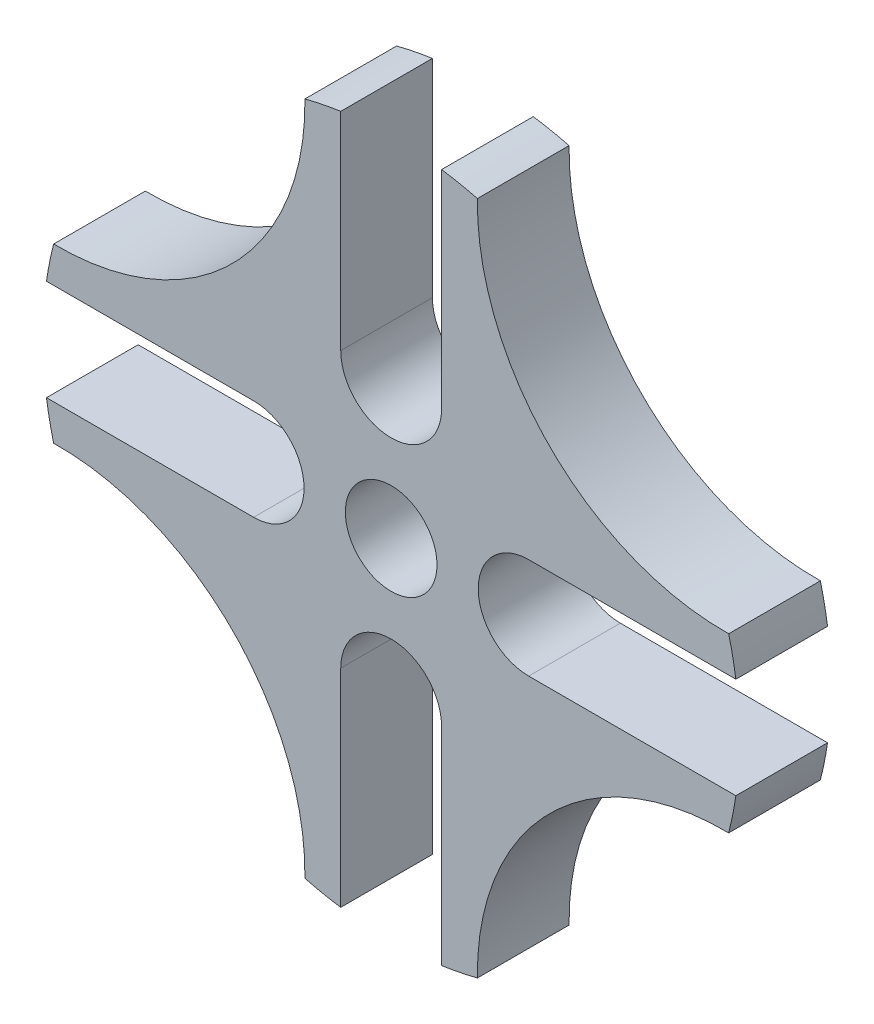
ISO-10303-21;
HEADER;
FILE_DESCRIPTION(('STEP AP214'),'2;1');
FILE_NAME('part.step','',(''),(''),'','','');
FILE_SCHEMA(('AUTOMOTIVE_DESIGN { 1 0 10303 214 1 1 1 1 }'));
ENDSEC;
DATA;
#1=APPLICATION_CONTEXT('core data for automotive mechanical design processes');
#2=APPLICATION_PROTOCOL_DEFINITION('international standard','automotive_design',2000,#1);
#3=PRODUCT_CONTEXT('',#1,'mechanical');
#4=PRODUCT('Part','Part','',(#3));
#5=PRODUCT_RELATED_PRODUCT_CATEGORY('part','',(#4));
#6=PRODUCT_DEFINITION_FORMATION('','',#4);
#7=PRODUCT_DEFINITION_CONTEXT('part definition',#1,'design');
#8=PRODUCT_DEFINITION('design','',#6,#7);
#9=PRODUCT_DEFINITION_SHAPE('','',#8);
#10=(LENGTH_UNIT() NAMED_UNIT(*) SI_UNIT(.MILLI.,.METRE.));
#11=(NAMED_UNIT(*) PLANE_ANGLE_UNIT() SI_UNIT($,.RADIAN.));
#12=(NAMED_UNIT(*) SI_UNIT($,.STERADIAN.) SOLID_ANGLE_UNIT());
#13=UNCERTAINTY_MEASURE_WITH_UNIT(LENGTH_MEASURE(1.E-05),#10,'distance_accuracy_value','');
#14=(GEOMETRIC_REPRESENTATION_CONTEXT(3) GLOBAL_UNCERTAINTY_ASSIGNED_CONTEXT((#13)) GLOBAL_UNIT_ASSIGNED_CONTEXT((#10,
#11,#12)) REPRESENTATION_CONTEXT('',''));
#15=CARTESIAN_POINT('',(0.,0.,0.));
#16=DIRECTION('',(0.,0.,1.));
#17=DIRECTION('',(1.,0.,0.));
#18=AXIS2_PLACEMENT_3D('',#15,#16,#17);
#19=CARTESIAN_POINT('',(0.,0.,10.));
#20=DIRECTION('',(0.,0.,1.));
#21=DIRECTION('',(1.,0.,0.));
#22=AXIS2_PLACEMENT_3D('',#19,#20,#21);
#23=PLANE('',#22);
#24=CARTESIAN_POINT('',(0.,0.,10.));
#25=DIRECTION('',(0.,0.,1.));
#26=DIRECTION('',(1.,0.,0.));
#27=AXIS2_PLACEMENT_3D('',#24,#25,#26);
#28=CIRCLE('',#27,38.);
#29=CARTESIAN_POINT('',(-9.40826438850213,-36.8169059155715,10.));
#30=VERTEX_POINT('',#29);
#31=CARTESIAN_POINT('',(-5.5,-37.5998670210414,10.));
#32=VERTEX_POINT('',#31);
#33=EDGE_CURVE('E276',#30,#32,#28,.T.);
#34=ORIENTED_EDGE('',*,*,#33,.T.);
#35=DIRECTION('',(0.,1.,0.));
#36=VECTOR('',#35,1.);
#37=CARTESIAN_POINT('',(-5.5,-15.,10.));
#38=LINE('',#37,#36);
#39=CARTESIAN_POINT('',(-5.5,-15.,10.));
#40=VERTEX_POINT('',#39);
#41=EDGE_CURVE('E150',#32,#40,#38,.T.);
#42=ORIENTED_EDGE('',*,*,#41,.T.);
#43=CARTESIAN_POINT('',(0.,-15.,10.));
#44=DIRECTION('',(0.,0.,-1.));
#45=DIRECTION('',(1.,0.,0.));
#46=AXIS2_PLACEMENT_3D('',#43,#44,#45);
#47=CIRCLE('',#46,5.5);
#48=CARTESIAN_POINT('',(5.5,-15.,10.));
#49=VERTEX_POINT('',#48);
#50=EDGE_CURVE('E345',#40,#49,#47,.T.);
#51=ORIENTED_EDGE('',*,*,#50,.T.);
#52=DIRECTION('',(0.,-1.,0.));
#53=VECTOR('',#52,1.);
#54=CARTESIAN_POINT('',(5.5,-15.,10.));
#55=LINE('',#54,#53);
#56=CARTESIAN_POINT('',(5.5,-37.5998670210414,10.));
#57=VERTEX_POINT('',#56);
#58=EDGE_CURVE('E363',#49,#57,#55,.T.);
#59=ORIENTED_EDGE('',*,*,#58,.T.);
#60=CARTESIAN_POINT('',(0.,0.,10.));
#61=DIRECTION('',(0.,0.,1.));
#62=DIRECTION('',(1.,0.,0.));
#63=AXIS2_PLACEMENT_3D('',#60,#61,#62);
#64=CIRCLE('',#63,38.);
#65=CARTESIAN_POINT('',(9.40826438850226,-36.8169059155714,10.));
#66=VERTEX_POINT('',#65);
#67=EDGE_CURVE('E356',#57,#66,#64,.T.);
#68=ORIENTED_EDGE('',*,*,#67,.T.);
#69=CARTESIAN_POINT('',(36.4051241273476,-36.4051241273475,10.));
#70=DIRECTION('',(0.,0.,-1.));
#71=DIRECTION('',(1.,0.,0.));
#72=AXIS2_PLACEMENT_3D('',#69,#70,#71);
#73=CIRCLE('',#72,27.);
#74=CARTESIAN_POINT('',(36.8169059155715,-9.40826438850214,10.));
#75=VERTEX_POINT('',#74);
#76=EDGE_CURVE('E357',#66,#75,#73,.T.);
#77=ORIENTED_EDGE('',*,*,#76,.T.);
#78=CARTESIAN_POINT('',(0.,0.,10.));
#79=DIRECTION('',(0.,0.,1.));
#80=DIRECTION('',(1.,0.,0.));
#81=AXIS2_PLACEMENT_3D('',#78,#79,#80);
#82=CIRCLE('',#81,38.);
#83=CARTESIAN_POINT('',(37.5998670210414,-5.5,10.));
#84=VERTEX_POINT('',#83);
#85=EDGE_CURVE('E361',#75,#84,#82,.T.);
#86=ORIENTED_EDGE('',*,*,#85,.T.);
#87=DIRECTION('',(-1.,0.,0.));
#88=VECTOR('',#87,1.);
#89=CARTESIAN_POINT('',(14.9999999999999,-5.50000000000016,10.));
#90=LINE('',#89,#88);
#91=CARTESIAN_POINT('',(14.9999999999999,-5.50000000000016,10.));
#92=VERTEX_POINT('',#91);
#93=EDGE_CURVE('E369',#84,#92,#90,.T.);
#94=ORIENTED_EDGE('',*,*,#93,.T.);
#95=CARTESIAN_POINT('',(15.,-1.57116660247941E-13,10.));
#96=DIRECTION('',(0.,0.,-1.));
#97=DIRECTION('',(1.,0.,0.));
#98=AXIS2_PLACEMENT_3D('',#95,#96,#97);
#99=CIRCLE('',#98,5.5);
#100=CARTESIAN_POINT('',(15.0000000000001,5.49999999999984,10.));
#101=VERTEX_POINT('',#100);
#102=EDGE_CURVE('E371',#92,#101,#99,.T.);
#103=ORIENTED_EDGE('',*,*,#102,.T.);
#104=DIRECTION('',(1.,0.,0.));
#105=VECTOR('',#104,1.);
#106=CARTESIAN_POINT('',(15.0000000000001,5.49999999999984,10.));
#107=LINE('',#106,#105);
#108=CARTESIAN_POINT('',(37.5998670210415,5.49999999999961,10.));
#109=VERTEX_POINT('',#108);
#110=EDGE_CURVE('E373',#101,#109,#107,.T.);
#111=ORIENTED_EDGE('',*,*,#110,.T.);
#112=CARTESIAN_POINT('',(0.,0.,10.));
#113=DIRECTION('',(0.,0.,1.));
#114=DIRECTION('',(1.,0.,0.));
#115=AXIS2_PLACEMENT_3D('',#112,#113,#114);
#116=CIRCLE('',#115,38.);
#117=CARTESIAN_POINT('',(36.8169059155714,9.40826438850227,10.));
#118=VERTEX_POINT('',#117);
#119=EDGE_CURVE('E374',#109,#118,#116,.T.);
#120=ORIENTED_EDGE('',*,*,#119,.T.);
#121=CARTESIAN_POINT('',(36.4051241273474,36.4051241273476,10.));
#122=DIRECTION('',(0.,0.,-1.));
#123=DIRECTION('',(1.,0.,0.));
#124=AXIS2_PLACEMENT_3D('',#121,#122,#123);
#125=CIRCLE('',#124,27.);
#126=CARTESIAN_POINT('',(9.40826438850214,36.8169059155715,10.));
#127=VERTEX_POINT('',#126);
#128=EDGE_CURVE('E380',#118,#127,#125,.T.);
#129=ORIENTED_EDGE('',*,*,#128,.T.);
#130=CARTESIAN_POINT('',(0.,0.,10.));
#131=DIRECTION('',(0.,0.,1.));
#132=DIRECTION('',(1.,0.,0.));
#133=AXIS2_PLACEMENT_3D('',#130,#131,#132);
#134=CIRCLE('',#133,38.);
#135=CARTESIAN_POINT('',(5.50000000000026,37.5998670210414,10.));
#136=VERTEX_POINT('',#135);
#137=EDGE_CURVE('E377',#127,#136,#134,.T.);
#138=ORIENTED_EDGE('',*,*,#137,.T.);
#139=DIRECTION('',(0.,-1.,0.));
#140=VECTOR('',#139,1.);
#141=CARTESIAN_POINT('',(5.5000000000001,15.,10.));
#142=LINE('',#141,#140);
#143=CARTESIAN_POINT('',(5.5000000000001,15.,10.));
#144=VERTEX_POINT('',#143);
#145=EDGE_CURVE('E381',#136,#144,#142,.T.);
#146=ORIENTED_EDGE('',*,*,#145,.T.);
#147=CARTESIAN_POINT('',(1.04744440165294E-13,15.,10.));
#148=DIRECTION('',(0.,0.,-1.));
#149=DIRECTION('',(1.,0.,0.));
#150=AXIS2_PLACEMENT_3D('',#147,#148,#149);
#151=CIRCLE('',#150,5.5);
#152=CARTESIAN_POINT('',(-5.49999999999989,15.,10.));
#153=VERTEX_POINT('',#152);
#154=EDGE_CURVE('E382',#144,#153,#151,.T.);
#155=ORIENTED_EDGE('',*,*,#154,.T.);
#156=DIRECTION('',(0.,1.,0.));
#157=VECTOR('',#156,1.);
#158=CARTESIAN_POINT('',(-5.49999999999989,15.,10.));
#159=LINE('',#158,#157);
#160=CARTESIAN_POINT('',(-5.49999999999974,37.5998670210415,10.));
#161=VERTEX_POINT('',#160);
#162=EDGE_CURVE('E384',#153,#161,#159,.T.);
#163=ORIENTED_EDGE('',*,*,#162,.T.);
#164=CARTESIAN_POINT('',(0.,0.,10.));
#165=DIRECTION('',(0.,0.,1.));
#166=DIRECTION('',(1.,0.,0.));
#167=AXIS2_PLACEMENT_3D('',#164,#165,#166);
#168=CIRCLE('',#167,38.);
#169=CARTESIAN_POINT('',(-9.40826438850228,36.8169059155714,10.));
#170=VERTEX_POINT('',#169);
#171=EDGE_CURVE('E390',#161,#170,#168,.T.);
#172=ORIENTED_EDGE('',*,*,#171,.T.);
#173=CARTESIAN_POINT('',(-36.4051241273476,36.4051241273475,10.));
#174=DIRECTION('',(0.,0.,-1.));
#175=DIRECTION('',(1.,0.,0.));
#176=AXIS2_PLACEMENT_3D('',#173,#174,#175);
#177=CIRCLE('',#176,27.);
#178=CARTESIAN_POINT('',(-36.8169059155715,9.40826438850215,10.));
#179=VERTEX_POINT('',#178);
#180=EDGE_CURVE('E386',#170,#179,#177,.T.);
#181=ORIENTED_EDGE('',*,*,#180,.T.);
#182=CARTESIAN_POINT('',(0.,0.,10.));
#183=DIRECTION('',(0.,0.,1.));
#184=DIRECTION('',(1.,0.,0.));
#185=AXIS2_PLACEMENT_3D('',#182,#183,#184);
#186=CIRCLE('',#185,38.);
#187=CARTESIAN_POINT('',(-37.5998670210414,5.50000000000013,10.));
#188=VERTEX_POINT('',#187);
#189=EDGE_CURVE('E392',#179,#188,#186,.T.);
#190=ORIENTED_EDGE('',*,*,#189,.T.);
#191=DIRECTION('',(1.,0.,0.));
#192=VECTOR('',#191,1.);
#193=CARTESIAN_POINT('',(-15.,5.50000000000005,10.));
#194=LINE('',#193,#192);
#195=CARTESIAN_POINT('',(-15.,5.50000000000005,10.));
#196=VERTEX_POINT('',#195);
#197=EDGE_CURVE('E394',#188,#196,#194,.T.);
#198=ORIENTED_EDGE('',*,*,#197,.T.);
#199=CARTESIAN_POINT('',(-15.,0.,10.));
#200=DIRECTION('',(0.,0.,-1.));
#201=DIRECTION('',(1.,0.,0.));
#202=AXIS2_PLACEMENT_3D('',#199,#200,#201);
#203=CIRCLE('',#202,5.5);
#204=CARTESIAN_POINT('',(-15.,-5.49999999999995,10.));
#205=VERTEX_POINT('',#204);
#206=EDGE_CURVE('E212',#196,#205,#203,.T.);
#207=ORIENTED_EDGE('',*,*,#206,.T.);
#208=DIRECTION('',(-1.,0.,0.));
#209=VECTOR('',#208,1.);
#210=CARTESIAN_POINT('',(-15.,-5.49999999999995,10.));
#211=LINE('',#210,#209);
#212=CARTESIAN_POINT('',(-37.5998670210415,-5.49999999999987,10.));
#213=VERTEX_POINT('',#212);
#214=EDGE_CURVE('E208',#205,#213,#211,.T.);
#215=ORIENTED_EDGE('',*,*,#214,.T.);
#216=CARTESIAN_POINT('',(0.,0.,10.));
#217=DIRECTION('',(0.,0.,1.));
#218=DIRECTION('',(1.,0.,0.));
#219=AXIS2_PLACEMENT_3D('',#216,#217,#218);
#220=CIRCLE('',#219,38.);
#221=CARTESIAN_POINT('',(-36.8169059155715,-9.40826438850228,10.));
#222=VERTEX_POINT('',#221);
#223=EDGE_CURVE('E215',#213,#222,#220,.T.);
#224=ORIENTED_EDGE('',*,*,#223,.T.);
#225=CARTESIAN_POINT('',(-36.4051241273474,-36.4051241273476,10.));
#226=DIRECTION('',(0.,0.,-1.));
#227=DIRECTION('',(1.,0.,0.));
#228=AXIS2_PLACEMENT_3D('',#225,#226,#227);
#229=CIRCLE('',#228,27.);
#230=EDGE_CURVE('E57',#222,#30,#229,.T.);
#231=ORIENTED_EDGE('',*,*,#230,.T.);
#232=EDGE_LOOP('',(#34,#42,#51,#59,#68,#77,#86,#94,#103,#111,#120,#129,#138,#146,#155,#163,#172,
#181,#190,#198,#207,#215,#224,#231));
#233=FACE_BOUND('',#232,.T.);
#234=CARTESIAN_POINT('',(0.,0.,10.));
#235=DIRECTION('',(0.,0.,1.));
#236=DIRECTION('',(1.,0.,0.));
#237=AXIS2_PLACEMENT_3D('',#234,#235,#236);
#238=CIRCLE('',#237,5.);
#239=CARTESIAN_POINT('',(5.,0.,10.));
#240=VERTEX_POINT('',#239);
#241=EDGE_CURVE('E237',#240,#240,#238,.T.);
#242=ORIENTED_EDGE('',*,*,#241,.F.);
#243=EDGE_LOOP('',(#242));
#244=FACE_BOUND('',#243,.T.);
#245=ADVANCED_FACE('F39',(#233,#244),#23,.T.);
#246=CARTESIAN_POINT('',(0.,0.,0.));
#247=DIRECTION('',(0.,0.,1.));
#248=DIRECTION('',(1.,0.,0.));
#249=AXIS2_PLACEMENT_3D('',#246,#247,#248);
#250=PLANE('',#249);
#251=CARTESIAN_POINT('',(0.,0.,0.));
#252=DIRECTION('',(0.,0.,1.));
#253=DIRECTION('',(1.,0.,0.));
#254=AXIS2_PLACEMENT_3D('',#251,#252,#253);
#255=CIRCLE('',#254,38.);
#256=CARTESIAN_POINT('',(-9.40826438850213,-36.8169059155715,0.));
#257=VERTEX_POINT('',#256);
#258=CARTESIAN_POINT('',(-5.5,-37.5998670210414,0.));
#259=VERTEX_POINT('',#258);
#260=EDGE_CURVE('E235',#257,#259,#255,.T.);
#261=ORIENTED_EDGE('',*,*,#260,.F.);
#262=CARTESIAN_POINT('',(-36.4051241273474,-36.4051241273476,0.));
#263=DIRECTION('',(0.,0.,-1.));
#264=DIRECTION('',(1.,0.,0.));
#265=AXIS2_PLACEMENT_3D('',#262,#263,#264);
#266=CIRCLE('',#265,27.);
#267=CARTESIAN_POINT('',(-36.8169059155715,-9.40826438850228,0.));
#268=VERTEX_POINT('',#267);
#269=EDGE_CURVE('E139',#268,#257,#266,.T.);
#270=ORIENTED_EDGE('',*,*,#269,.F.);
#271=CARTESIAN_POINT('',(0.,0.,0.));
#272=DIRECTION('',(0.,0.,1.));
#273=DIRECTION('',(1.,0.,0.));
#274=AXIS2_PLACEMENT_3D('',#271,#272,#273);
#275=CIRCLE('',#274,38.);
#276=CARTESIAN_POINT('',(-37.5998670210415,-5.49999999999987,0.));
#277=VERTEX_POINT('',#276);
#278=EDGE_CURVE('E134',#277,#268,#275,.T.);
#279=ORIENTED_EDGE('',*,*,#278,.F.);
#280=DIRECTION('',(-1.,0.,0.));
#281=VECTOR('',#280,1.);
#282=CARTESIAN_POINT('',(-15.,-5.49999999999995,0.));
#283=LINE('',#282,#281);
#284=CARTESIAN_POINT('',(-15.,-5.49999999999995,0.));
#285=VERTEX_POINT('',#284);
#286=EDGE_CURVE('E225',#285,#277,#283,.T.);
#287=ORIENTED_EDGE('',*,*,#286,.F.);
#288=CARTESIAN_POINT('',(-15.,0.,0.));
#289=DIRECTION('',(0.,0.,-1.));
#290=DIRECTION('',(1.,0.,0.));
#291=AXIS2_PLACEMENT_3D('',#288,#289,#290);
#292=CIRCLE('',#291,5.5);
#293=CARTESIAN_POINT('',(-15.,5.50000000000005,0.));
#294=VERTEX_POINT('',#293);
#295=EDGE_CURVE('E273',#294,#285,#292,.T.);
#296=ORIENTED_EDGE('',*,*,#295,.F.);
#297=DIRECTION('',(1.,0.,0.));
#298=VECTOR('',#297,1.);
#299=CARTESIAN_POINT('',(-15.,5.50000000000005,0.));
#300=LINE('',#299,#298);
#301=CARTESIAN_POINT('',(-37.5998670210414,5.50000000000013,0.));
#302=VERTEX_POINT('',#301);
#303=EDGE_CURVE('E275',#302,#294,#300,.T.);
#304=ORIENTED_EDGE('',*,*,#303,.F.);
#305=CARTESIAN_POINT('',(0.,0.,0.));
#306=DIRECTION('',(0.,0.,1.));
#307=DIRECTION('',(1.,0.,0.));
#308=AXIS2_PLACEMENT_3D('',#305,#306,#307);
#309=CIRCLE('',#308,38.);
#310=CARTESIAN_POINT('',(-36.8169059155715,9.40826438850215,0.));
#311=VERTEX_POINT('',#310);
#312=EDGE_CURVE('E269',#311,#302,#309,.T.);
#313=ORIENTED_EDGE('',*,*,#312,.F.);
#314=CARTESIAN_POINT('',(-36.4051241273476,36.4051241273475,0.));
#315=DIRECTION('',(0.,0.,-1.));
#316=DIRECTION('',(1.,0.,0.));
#317=AXIS2_PLACEMENT_3D('',#314,#315,#316);
#318=CIRCLE('',#317,27.);
#319=CARTESIAN_POINT('',(-9.40826438850228,36.8169059155714,0.));
#320=VERTEX_POINT('',#319);
#321=EDGE_CURVE('E268',#320,#311,#318,.T.);
#322=ORIENTED_EDGE('',*,*,#321,.F.);
#323=CARTESIAN_POINT('',(0.,0.,0.));
#324=DIRECTION('',(0.,0.,1.));
#325=DIRECTION('',(1.,0.,0.));
#326=AXIS2_PLACEMENT_3D('',#323,#324,#325);
#327=CIRCLE('',#326,38.);
#328=CARTESIAN_POINT('',(-5.49999999999974,37.5998670210415,0.));
#329=VERTEX_POINT('',#328);
#330=EDGE_CURVE('E266',#329,#320,#327,.T.);
#331=ORIENTED_EDGE('',*,*,#330,.F.);
#332=DIRECTION('',(0.,1.,0.));
#333=VECTOR('',#332,1.);
#334=CARTESIAN_POINT('',(-5.49999999999989,15.,0.));
#335=LINE('',#334,#333);
#336=CARTESIAN_POINT('',(-5.49999999999989,15.,0.));
#337=VERTEX_POINT('',#336);
#338=EDGE_CURVE('E262',#337,#329,#335,.T.);
#339=ORIENTED_EDGE('',*,*,#338,.F.);
#340=CARTESIAN_POINT('',(1.04744440165294E-13,15.,0.));
#341=DIRECTION('',(0.,0.,-1.));
#342=DIRECTION('',(1.,0.,0.));
#343=AXIS2_PLACEMENT_3D('',#340,#341,#342);
#344=CIRCLE('',#343,5.5);
#345=CARTESIAN_POINT('',(5.5000000000001,15.,0.));
#346=VERTEX_POINT('',#345);
#347=EDGE_CURVE('E265',#346,#337,#344,.T.);
#348=ORIENTED_EDGE('',*,*,#347,.F.);
#349=DIRECTION('',(0.,-1.,0.));
#350=VECTOR('',#349,1.);
#351=CARTESIAN_POINT('',(5.5000000000001,15.,0.));
#352=LINE('',#351,#350);
#353=CARTESIAN_POINT('',(5.50000000000026,37.5998670210414,0.));
#354=VERTEX_POINT('',#353);
#355=EDGE_CURVE('E257',#354,#346,#352,.T.);
#356=ORIENTED_EDGE('',*,*,#355,.F.);
#357=CARTESIAN_POINT('',(0.,0.,0.));
#358=DIRECTION('',(0.,0.,1.));
#359=DIRECTION('',(1.,0.,0.));
#360=AXIS2_PLACEMENT_3D('',#357,#358,#359);
#361=CIRCLE('',#360,38.);
#362=CARTESIAN_POINT('',(9.40826438850214,36.8169059155715,0.));
#363=VERTEX_POINT('',#362);
#364=EDGE_CURVE('E256',#363,#354,#361,.T.);
#365=ORIENTED_EDGE('',*,*,#364,.F.);
#366=CARTESIAN_POINT('',(36.4051241273474,36.4051241273476,0.));
#367=DIRECTION('',(0.,0.,-1.));
#368=DIRECTION('',(1.,0.,0.));
#369=AXIS2_PLACEMENT_3D('',#366,#367,#368);
#370=CIRCLE('',#369,27.);
#371=CARTESIAN_POINT('',(36.8169059155714,9.40826438850227,0.));
#372=VERTEX_POINT('',#371);
#373=EDGE_CURVE('E258',#372,#363,#370,.T.);
#374=ORIENTED_EDGE('',*,*,#373,.F.);
#375=CARTESIAN_POINT('',(0.,0.,0.));
#376=DIRECTION('',(0.,0.,1.));
#377=DIRECTION('',(1.,0.,0.));
#378=AXIS2_PLACEMENT_3D('',#375,#376,#377);
#379=CIRCLE('',#378,38.);
#380=CARTESIAN_POINT('',(37.5998670210415,5.49999999999961,0.));
#381=VERTEX_POINT('',#380);
#382=EDGE_CURVE('E255',#381,#372,#379,.T.);
#383=ORIENTED_EDGE('',*,*,#382,.F.);
#384=DIRECTION('',(1.,0.,0.));
#385=VECTOR('',#384,1.);
#386=CARTESIAN_POINT('',(15.0000000000001,5.49999999999984,0.));
#387=LINE('',#386,#385);
#388=CARTESIAN_POINT('',(15.0000000000001,5.49999999999984,0.));
#389=VERTEX_POINT('',#388);
#390=EDGE_CURVE('E252',#389,#381,#387,.T.);
#391=ORIENTED_EDGE('',*,*,#390,.F.);
#392=CARTESIAN_POINT('',(15.,-1.57116660247941E-13,0.));
#393=DIRECTION('',(0.,0.,-1.));
#394=DIRECTION('',(1.,0.,0.));
#395=AXIS2_PLACEMENT_3D('',#392,#393,#394);
#396=CIRCLE('',#395,5.5);
#397=CARTESIAN_POINT('',(14.9999999999999,-5.50000000000016,0.));
#398=VERTEX_POINT('',#397);
#399=EDGE_CURVE('E247',#398,#389,#396,.T.);
#400=ORIENTED_EDGE('',*,*,#399,.F.);
#401=DIRECTION('',(-1.,0.,0.));
#402=VECTOR('',#401,1.);
#403=CARTESIAN_POINT('',(14.9999999999999,-5.50000000000016,0.));
#404=LINE('',#403,#402);
#405=CARTESIAN_POINT('',(37.5998670210414,-5.5,0.));
#406=VERTEX_POINT('',#405);
#407=EDGE_CURVE('E246',#406,#398,#404,.T.);
#408=ORIENTED_EDGE('',*,*,#407,.F.);
#409=CARTESIAN_POINT('',(0.,0.,0.));
#410=DIRECTION('',(0.,0.,1.));
#411=DIRECTION('',(1.,0.,0.));
#412=AXIS2_PLACEMENT_3D('',#409,#410,#411);
#413=CIRCLE('',#412,38.);
#414=CARTESIAN_POINT('',(36.8169059155715,-9.40826438850214,0.));
#415=VERTEX_POINT('',#414);
#416=EDGE_CURVE('E248',#415,#406,#413,.T.);
#417=ORIENTED_EDGE('',*,*,#416,.F.);
#418=CARTESIAN_POINT('',(36.4051241273476,-36.4051241273475,0.));
#419=DIRECTION('',(0.,0.,-1.));
#420=DIRECTION('',(1.,0.,0.));
#421=AXIS2_PLACEMENT_3D('',#418,#419,#420);
#422=CIRCLE('',#421,27.);
#423=CARTESIAN_POINT('',(9.40826438850226,-36.8169059155714,0.));
#424=VERTEX_POINT('',#423);
#425=EDGE_CURVE('E241',#424,#415,#422,.T.);
#426=ORIENTED_EDGE('',*,*,#425,.F.);
#427=CARTESIAN_POINT('',(0.,0.,0.));
#428=DIRECTION('',(0.,0.,1.));
#429=DIRECTION('',(1.,0.,0.));
#430=AXIS2_PLACEMENT_3D('',#427,#428,#429);
#431=CIRCLE('',#430,38.);
#432=CARTESIAN_POINT('',(5.5,-37.5998670210414,0.));
#433=VERTEX_POINT('',#432);
#434=EDGE_CURVE('E245',#433,#424,#431,.T.);
#435=ORIENTED_EDGE('',*,*,#434,.F.);
#436=DIRECTION('',(0.,-1.,0.));
#437=VECTOR('',#436,1.);
#438=CARTESIAN_POINT('',(5.5,-15.,0.));
#439=LINE('',#438,#437);
#440=CARTESIAN_POINT('',(5.5,-15.,0.));
#441=VERTEX_POINT('',#440);
#442=EDGE_CURVE('E238',#441,#433,#439,.T.);
#443=ORIENTED_EDGE('',*,*,#442,.F.);
#444=CARTESIAN_POINT('',(0.,-15.,0.));
#445=DIRECTION('',(0.,0.,-1.));
#446=DIRECTION('',(1.,0.,0.));
#447=AXIS2_PLACEMENT_3D('',#444,#445,#446);
#448=CIRCLE('',#447,5.5);
#449=CARTESIAN_POINT('',(-5.5,-15.,0.));
#450=VERTEX_POINT('',#449);
#451=EDGE_CURVE('E236',#450,#441,#448,.T.);
#452=ORIENTED_EDGE('',*,*,#451,.F.);
#453=DIRECTION('',(0.,1.,0.));
#454=VECTOR('',#453,1.);
#455=CARTESIAN_POINT('',(-5.5,-15.,0.));
#456=LINE('',#455,#454);
#457=EDGE_CURVE('E232',#259,#450,#456,.T.);
#458=ORIENTED_EDGE('',*,*,#457,.F.);
#459=EDGE_LOOP('',(#261,#270,#279,#287,#296,#304,#313,#322,#331,#339,#348,#356,#365,#374,#383,
#391,#400,#408,#417,#426,#435,#443,#452,#458));
#460=FACE_BOUND('',#459,.T.);
#461=CARTESIAN_POINT('',(0.,0.,0.));
#462=DIRECTION('',(0.,0.,1.));
#463=DIRECTION('',(1.,0.,0.));
#464=AXIS2_PLACEMENT_3D('',#461,#462,#463);
#465=CIRCLE('',#464,5.);
#466=CARTESIAN_POINT('',(5.,0.,0.));
#467=VERTEX_POINT('',#466);
#468=EDGE_CURVE('E698',#467,#467,#465,.T.);
#469=ORIENTED_EDGE('',*,*,#468,.T.);
#470=EDGE_LOOP('',(#469));
#471=FACE_BOUND('',#470,.T.);
#472=ADVANCED_FACE('F347',(#460,#471),#250,.F.);
#473=CARTESIAN_POINT('',(0.,0.,10.));
#474=DIRECTION('',(0.,0.,-1.));
#475=DIRECTION('',(-1.,0.,0.));
#476=AXIS2_PLACEMENT_3D('',#473,#474,#475);
#477=CYLINDRICAL_SURFACE('',#476,38.);
#478=ORIENTED_EDGE('',*,*,#260,.T.);
#479=DIRECTION('',(0.,0.,-1.));
#480=VECTOR('',#479,1.);
#481=CARTESIAN_POINT('',(-5.5,-37.5998670210414,10.));
#482=LINE('',#481,#480);
#483=EDGE_CURVE('E11',#32,#259,#482,.T.);
#484=ORIENTED_EDGE('',*,*,#483,.F.);
#485=ORIENTED_EDGE('',*,*,#33,.F.);
#486=DIRECTION('',(0.,0.,-1.));
#487=VECTOR('',#486,1.);
#488=CARTESIAN_POINT('',(-9.40826438850213,-36.8169059155715,10.));
#489=LINE('',#488,#487);
#490=EDGE_CURVE('E229',#30,#257,#489,.T.);
#491=ORIENTED_EDGE('',*,*,#490,.T.);
#492=EDGE_LOOP('',(#478,#484,#485,#491));
#493=FACE_BOUND('',#492,.T.);
#494=ADVANCED_FACE('F41',(#493),#477,.T.);
#495=CARTESIAN_POINT('',(-5.5,-15.,10.));
#496=DIRECTION('',(-1.,0.,0.));
#497=DIRECTION('',(0.,-1.,0.));
#498=AXIS2_PLACEMENT_3D('',#495,#496,#497);
#499=PLANE('',#498);
#500=ORIENTED_EDGE('',*,*,#457,.T.);
#501=DIRECTION('',(0.,0.,-1.));
#502=VECTOR('',#501,1.);
#503=CARTESIAN_POINT('',(-5.5,-15.,10.));
#504=LINE('',#503,#502);
#505=EDGE_CURVE('E48',#40,#450,#504,.T.);
#506=ORIENTED_EDGE('',*,*,#505,.F.);
#507=ORIENTED_EDGE('',*,*,#41,.F.);
#508=ORIENTED_EDGE('',*,*,#483,.T.);
#509=EDGE_LOOP('',(#500,#506,#507,#508));
#510=FACE_BOUND('',#509,.T.);
#511=ADVANCED_FACE('F430',(#510),#499,.F.);
#512=CARTESIAN_POINT('',(0.,-15.,10.));
#513=DIRECTION('',(0.,0.,-1.));
#514=DIRECTION('',(-1.,0.,0.));
#515=AXIS2_PLACEMENT_3D('',#512,#513,#514);
#516=CYLINDRICAL_SURFACE('',#515,5.5);
#517=ORIENTED_EDGE('',*,*,#451,.T.);
#518=DIRECTION('',(0.,0.,-1.));
#519=VECTOR('',#518,1.);
#520=CARTESIAN_POINT('',(5.5,-15.,10.));
#521=LINE('',#520,#519);
#522=EDGE_CURVE('E331',#49,#441,#521,.T.);
#523=ORIENTED_EDGE('',*,*,#522,.F.);
#524=ORIENTED_EDGE('',*,*,#50,.F.);
#525=ORIENTED_EDGE('',*,*,#505,.T.);
#526=EDGE_LOOP('',(#517,#523,#524,#525));
#527=FACE_BOUND('',#526,.T.);
#528=ADVANCED_FACE('F338',(#527),#516,.F.);
#529=CARTESIAN_POINT('',(5.5,-15.,10.));
#530=DIRECTION('',(1.,0.,0.));
#531=DIRECTION('',(0.,0.,-1.));
#532=AXIS2_PLACEMENT_3D('',#529,#530,#531);
#533=PLANE('',#532);
#534=ORIENTED_EDGE('',*,*,#442,.T.);
#535=DIRECTION('',(0.,0.,-1.));
#536=VECTOR('',#535,1.);
#537=CARTESIAN_POINT('',(5.5,-37.5998670210414,10.));
#538=LINE('',#537,#536);
#539=EDGE_CURVE('E332',#57,#433,#538,.T.);
#540=ORIENTED_EDGE('',*,*,#539,.F.);
#541=ORIENTED_EDGE('',*,*,#58,.F.);
#542=ORIENTED_EDGE('',*,*,#522,.T.);
#543=EDGE_LOOP('',(#534,#540,#541,#542));
#544=FACE_BOUND('',#543,.T.);
#545=ADVANCED_FACE('F355',(#544),#533,.F.);
#546=CARTESIAN_POINT('',(0.,0.,10.));
#547=DIRECTION('',(0.,0.,-1.));
#548=DIRECTION('',(-1.,0.,0.));
#549=AXIS2_PLACEMENT_3D('',#546,#547,#548);
#550=CYLINDRICAL_SURFACE('',#549,38.);
#551=ORIENTED_EDGE('',*,*,#434,.T.);
#552=DIRECTION('',(0.,0.,-1.));
#553=VECTOR('',#552,1.);
#554=CARTESIAN_POINT('',(9.40826438850226,-36.8169059155714,10.));
#555=LINE('',#554,#553);
#556=EDGE_CURVE('E327',#66,#424,#555,.T.);
#557=ORIENTED_EDGE('',*,*,#556,.F.);
#558=ORIENTED_EDGE('',*,*,#67,.F.);
#559=ORIENTED_EDGE('',*,*,#539,.T.);
#560=EDGE_LOOP('',(#551,#557,#558,#559));
#561=FACE_BOUND('',#560,.T.);
#562=ADVANCED_FACE('F358',(#561),#550,.T.);
#563=CARTESIAN_POINT('',(36.4051241273476,-36.4051241273475,10.));
#564=DIRECTION('',(0.,0.,-1.));
#565=DIRECTION('',(-1.,0.,0.));
#566=AXIS2_PLACEMENT_3D('',#563,#564,#565);
#567=CYLINDRICAL_SURFACE('',#566,27.);
#568=ORIENTED_EDGE('',*,*,#425,.T.);
#569=DIRECTION('',(0.,0.,-1.));
#570=VECTOR('',#569,1.);
#571=CARTESIAN_POINT('',(36.8169059155715,-9.40826438850214,10.));
#572=LINE('',#571,#570);
#573=EDGE_CURVE('E324',#75,#415,#572,.T.);
#574=ORIENTED_EDGE('',*,*,#573,.F.);
#575=ORIENTED_EDGE('',*,*,#76,.F.);
#576=ORIENTED_EDGE('',*,*,#556,.T.);
#577=EDGE_LOOP('',(#568,#574,#575,#576));
#578=FACE_BOUND('',#577,.T.);
#579=ADVANCED_FACE('F439',(#578),#567,.F.);
#580=CARTESIAN_POINT('',(0.,0.,10.));
#581=DIRECTION('',(0.,0.,-1.));
#582=DIRECTION('',(-1.,0.,0.));
#583=AXIS2_PLACEMENT_3D('',#580,#581,#582);
#584=CYLINDRICAL_SURFACE('',#583,38.);
#585=ORIENTED_EDGE('',*,*,#416,.T.);
#586=DIRECTION('',(0.,0.,-1.));
#587=VECTOR('',#586,1.);
#588=CARTESIAN_POINT('',(37.5998670210414,-5.5,10.));
#589=LINE('',#588,#587);
#590=EDGE_CURVE('E325',#84,#406,#589,.T.);
#591=ORIENTED_EDGE('',*,*,#590,.F.);
#592=ORIENTED_EDGE('',*,*,#85,.F.);
#593=ORIENTED_EDGE('',*,*,#573,.T.);
#594=EDGE_LOOP('',(#585,#591,#592,#593));
#595=FACE_BOUND('',#594,.T.);
#596=ADVANCED_FACE('F444',(#595),#584,.T.);
#597=CARTESIAN_POINT('',(14.9999999999999,-5.50000000000016,10.));
#598=DIRECTION('',(0.,-1.,0.));
#599=DIRECTION('',(1.,0.,0.));
#600=AXIS2_PLACEMENT_3D('',#597,#598,#599);
#601=PLANE('',#600);
#602=ORIENTED_EDGE('',*,*,#407,.T.);
#603=DIRECTION('',(0.,0.,-1.));
#604=VECTOR('',#603,1.);
#605=CARTESIAN_POINT('',(14.9999999999999,-5.50000000000016,10.));
#606=LINE('',#605,#604);
#607=EDGE_CURVE('E317',#92,#398,#606,.T.);
#608=ORIENTED_EDGE('',*,*,#607,.F.);
#609=ORIENTED_EDGE('',*,*,#93,.F.);
#610=ORIENTED_EDGE('',*,*,#590,.T.);
#611=EDGE_LOOP('',(#602,#608,#609,#610));
#612=FACE_BOUND('',#611,.T.);
#613=ADVANCED_FACE('F450',(#612),#601,.F.);
#614=CARTESIAN_POINT('',(15.,-1.57116660247941E-13,10.));
#615=DIRECTION('',(0.,0.,-1.));
#616=DIRECTION('',(-1.,0.,0.));
#617=AXIS2_PLACEMENT_3D('',#614,#615,#616);
#618=CYLINDRICAL_SURFACE('',#617,5.5);
#619=ORIENTED_EDGE('',*,*,#399,.T.);
#620=DIRECTION('',(0.,0.,-1.));
#621=VECTOR('',#620,1.);
#622=CARTESIAN_POINT('',(15.0000000000001,5.49999999999984,10.));
#623=LINE('',#622,#621);
#624=EDGE_CURVE('E316',#101,#389,#623,.T.);
#625=ORIENTED_EDGE('',*,*,#624,.F.);
#626=ORIENTED_EDGE('',*,*,#102,.F.);
#627=ORIENTED_EDGE('',*,*,#607,.T.);
#628=EDGE_LOOP('',(#619,#625,#626,#627));
#629=FACE_BOUND('',#628,.T.);
#630=ADVANCED_FACE('F453',(#629),#618,.F.);
#631=CARTESIAN_POINT('',(15.0000000000001,5.49999999999984,10.));
#632=DIRECTION('',(0.,1.,0.));
#633=DIRECTION('',(-1.,0.,0.));
#634=AXIS2_PLACEMENT_3D('',#631,#632,#633);
#635=PLANE('',#634);
#636=ORIENTED_EDGE('',*,*,#390,.T.);
#637=DIRECTION('',(0.,0.,-1.));
#638=VECTOR('',#637,1.);
#639=CARTESIAN_POINT('',(37.5998670210415,5.49999999999961,10.));
#640=LINE('',#639,#638);
#641=EDGE_CURVE('E311',#109,#381,#640,.T.);
#642=ORIENTED_EDGE('',*,*,#641,.F.);
#643=ORIENTED_EDGE('',*,*,#110,.F.);
#644=ORIENTED_EDGE('',*,*,#624,.T.);
#645=EDGE_LOOP('',(#636,#642,#643,#644));
#646=FACE_BOUND('',#645,.T.);
#647=ADVANCED_FACE('F452',(#646),#635,.F.);
#648=CARTESIAN_POINT('',(0.,0.,10.));
#649=DIRECTION('',(0.,0.,-1.));
#650=DIRECTION('',(-1.,0.,0.));
#651=AXIS2_PLACEMENT_3D('',#648,#649,#650);
#652=CYLINDRICAL_SURFACE('',#651,38.);
#653=ORIENTED_EDGE('',*,*,#382,.T.);
#654=DIRECTION('',(0.,0.,-1.));
#655=VECTOR('',#654,1.);
#656=CARTESIAN_POINT('',(36.8169059155714,9.40826438850227,10.));
#657=LINE('',#656,#655);
#658=EDGE_CURVE('E309',#118,#372,#657,.T.);
#659=ORIENTED_EDGE('',*,*,#658,.F.);
#660=ORIENTED_EDGE('',*,*,#119,.F.);
#661=ORIENTED_EDGE('',*,*,#641,.T.);
#662=EDGE_LOOP('',(#653,#659,#660,#661));
#663=FACE_BOUND('',#662,.T.);
#664=ADVANCED_FACE('F459',(#663),#652,.T.);
#665=CARTESIAN_POINT('',(36.4051241273474,36.4051241273476,10.));
#666=DIRECTION('',(0.,0.,-1.));
#667=DIRECTION('',(-1.,0.,0.));
#668=AXIS2_PLACEMENT_3D('',#665,#666,#667);
#669=CYLINDRICAL_SURFACE('',#668,27.);
#670=ORIENTED_EDGE('',*,*,#373,.T.);
#671=DIRECTION('',(0.,0.,-1.));
#672=VECTOR('',#671,1.);
#673=CARTESIAN_POINT('',(9.40826438850214,36.8169059155715,10.));
#674=LINE('',#673,#672);
#675=EDGE_CURVE('E307',#127,#363,#674,.T.);
#676=ORIENTED_EDGE('',*,*,#675,.F.);
#677=ORIENTED_EDGE('',*,*,#128,.F.);
#678=ORIENTED_EDGE('',*,*,#658,.T.);
#679=EDGE_LOOP('',(#670,#676,#677,#678));
#680=FACE_BOUND('',#679,.T.);
#681=ADVANCED_FACE('F464',(#680),#669,.F.);
#682=CARTESIAN_POINT('',(0.,0.,10.));
#683=DIRECTION('',(0.,0.,-1.));
#684=DIRECTION('',(-1.,0.,0.));
#685=AXIS2_PLACEMENT_3D('',#682,#683,#684);
#686=CYLINDRICAL_SURFACE('',#685,38.);
#687=ORIENTED_EDGE('',*,*,#364,.T.);
#688=DIRECTION('',(0.,0.,-1.));
#689=VECTOR('',#688,1.);
#690=CARTESIAN_POINT('',(5.50000000000026,37.5998670210414,10.));
#691=LINE('',#690,#689);
#692=EDGE_CURVE('E304',#136,#354,#691,.T.);
#693=ORIENTED_EDGE('',*,*,#692,.F.);
#694=ORIENTED_EDGE('',*,*,#137,.F.);
#695=ORIENTED_EDGE('',*,*,#675,.T.);
#696=EDGE_LOOP('',(#687,#693,#694,#695));
#697=FACE_BOUND('',#696,.T.);
#698=ADVANCED_FACE('F470',(#697),#686,.T.);
#699=CARTESIAN_POINT('',(5.5000000000001,15.,10.));
#700=DIRECTION('',(1.,0.,0.));
#701=DIRECTION('',(0.,1.,0.));
#702=AXIS2_PLACEMENT_3D('',#699,#700,#701);
#703=PLANE('',#702);
#704=ORIENTED_EDGE('',*,*,#355,.T.);
#705=DIRECTION('',(0.,0.,-1.));
#706=VECTOR('',#705,1.);
#707=CARTESIAN_POINT('',(5.5000000000001,15.,10.));
#708=LINE('',#707,#706);
#709=EDGE_CURVE('E303',#144,#346,#708,.T.);
#710=ORIENTED_EDGE('',*,*,#709,.F.);
#711=ORIENTED_EDGE('',*,*,#145,.F.);
#712=ORIENTED_EDGE('',*,*,#692,.T.);
#713=EDGE_LOOP('',(#704,#710,#711,#712));
#714=FACE_BOUND('',#713,.T.);
#715=ADVANCED_FACE('F473',(#714),#703,.F.);
#716=CARTESIAN_POINT('',(1.04744440165294E-13,15.,10.));
#717=DIRECTION('',(0.,0.,-1.));
#718=DIRECTION('',(-1.,0.,0.));
#719=AXIS2_PLACEMENT_3D('',#716,#717,#718);
#720=CYLINDRICAL_SURFACE('',#719,5.5);
#721=ORIENTED_EDGE('',*,*,#347,.T.);
#722=DIRECTION('',(0.,0.,-1.));
#723=VECTOR('',#722,1.);
#724=CARTESIAN_POINT('',(-5.49999999999989,15.,10.));
#725=LINE('',#724,#723);
#726=EDGE_CURVE('E299',#153,#337,#725,.T.);
#727=ORIENTED_EDGE('',*,*,#726,.F.);
#728=ORIENTED_EDGE('',*,*,#154,.F.);
#729=ORIENTED_EDGE('',*,*,#709,.T.);
#730=EDGE_LOOP('',(#721,#727,#728,#729));
#731=FACE_BOUND('',#730,.T.);
#732=ADVANCED_FACE('F474',(#731),#720,.F.);
#733=CARTESIAN_POINT('',(-5.49999999999989,15.,10.));
#734=DIRECTION('',(-1.,0.,0.));
#735=DIRECTION('',(0.,-1.,0.));
#736=AXIS2_PLACEMENT_3D('',#733,#734,#735);
#737=PLANE('',#736);
#738=ORIENTED_EDGE('',*,*,#338,.T.);
#739=DIRECTION('',(0.,0.,-1.));
#740=VECTOR('',#739,1.);
#741=CARTESIAN_POINT('',(-5.49999999999974,37.5998670210415,10.));
#742=LINE('',#741,#740);
#743=EDGE_CURVE('E293',#161,#329,#742,.T.);
#744=ORIENTED_EDGE('',*,*,#743,.F.);
#745=ORIENTED_EDGE('',*,*,#162,.F.);
#746=ORIENTED_EDGE('',*,*,#726,.T.);
#747=EDGE_LOOP('',(#738,#744,#745,#746));
#748=FACE_BOUND('',#747,.T.);
#749=ADVANCED_FACE('F479',(#748),#737,.F.);
#750=CARTESIAN_POINT('',(0.,0.,10.));
#751=DIRECTION('',(0.,0.,-1.));
#752=DIRECTION('',(-1.,0.,0.));
#753=AXIS2_PLACEMENT_3D('',#750,#751,#752);
#754=CYLINDRICAL_SURFACE('',#753,38.);
#755=ORIENTED_EDGE('',*,*,#330,.T.);
#756=DIRECTION('',(0.,0.,-1.));
#757=VECTOR('',#756,1.);
#758=CARTESIAN_POINT('',(-9.40826438850228,36.8169059155714,10.));
#759=LINE('',#758,#757);
#760=EDGE_CURVE('E295',#170,#320,#759,.T.);
#761=ORIENTED_EDGE('',*,*,#760,.F.);
#762=ORIENTED_EDGE('',*,*,#171,.F.);
#763=ORIENTED_EDGE('',*,*,#743,.T.);
#764=EDGE_LOOP('',(#755,#761,#762,#763));
#765=FACE_BOUND('',#764,.T.);
#766=ADVANCED_FACE('F483',(#765),#754,.T.);
#767=CARTESIAN_POINT('',(-36.4051241273476,36.4051241273475,10.));
#768=DIRECTION('',(0.,0.,-1.));
#769=DIRECTION('',(-1.,0.,0.));
#770=AXIS2_PLACEMENT_3D('',#767,#768,#769);
#771=CYLINDRICAL_SURFACE('',#770,27.);
#772=ORIENTED_EDGE('',*,*,#321,.T.);
#773=DIRECTION('',(0.,0.,-1.));
#774=VECTOR('',#773,1.);
#775=CARTESIAN_POINT('',(-36.8169059155715,9.40826438850215,10.));
#776=LINE('',#775,#774);
#777=EDGE_CURVE('E289',#179,#311,#776,.T.);
#778=ORIENTED_EDGE('',*,*,#777,.F.);
#779=ORIENTED_EDGE('',*,*,#180,.F.);
#780=ORIENTED_EDGE('',*,*,#760,.T.);
#781=EDGE_LOOP('',(#772,#778,#779,#780));
#782=FACE_BOUND('',#781,.T.);
#783=ADVANCED_FACE('F490',(#782),#771,.F.);
#784=CARTESIAN_POINT('',(0.,0.,10.));
#785=DIRECTION('',(0.,0.,-1.));
#786=DIRECTION('',(-1.,0.,0.));
#787=AXIS2_PLACEMENT_3D('',#784,#785,#786);
#788=CYLINDRICAL_SURFACE('',#787,38.);
#789=ORIENTED_EDGE('',*,*,#312,.T.);
#790=DIRECTION('',(0.,0.,-1.));
#791=VECTOR('',#790,1.);
#792=CARTESIAN_POINT('',(-37.5998670210414,5.50000000000013,10.));
#793=LINE('',#792,#791);
#794=EDGE_CURVE('E288',#188,#302,#793,.T.);
#795=ORIENTED_EDGE('',*,*,#794,.F.);
#796=ORIENTED_EDGE('',*,*,#189,.F.);
#797=ORIENTED_EDGE('',*,*,#777,.T.);
#798=EDGE_LOOP('',(#789,#795,#796,#797));
#799=FACE_BOUND('',#798,.T.);
#800=ADVANCED_FACE('F491',(#799),#788,.T.);
#801=CARTESIAN_POINT('',(-15.,5.50000000000005,10.));
#802=DIRECTION('',(0.,1.,0.));
#803=DIRECTION('',(-1.,0.,0.));
#804=AXIS2_PLACEMENT_3D('',#801,#802,#803);
#805=PLANE('',#804);
#806=ORIENTED_EDGE('',*,*,#303,.T.);
#807=DIRECTION('',(0.,0.,-1.));
#808=VECTOR('',#807,1.);
#809=CARTESIAN_POINT('',(-15.,5.50000000000005,10.));
#810=LINE('',#809,#808);
#811=EDGE_CURVE('E284',#196,#294,#810,.T.);
#812=ORIENTED_EDGE('',*,*,#811,.F.);
#813=ORIENTED_EDGE('',*,*,#197,.F.);
#814=ORIENTED_EDGE('',*,*,#794,.T.);
#815=EDGE_LOOP('',(#806,#812,#813,#814));
#816=FACE_BOUND('',#815,.T.);
#817=ADVANCED_FACE('F399',(#816),#805,.F.);
#818=CARTESIAN_POINT('',(-15.,0.,10.));
#819=DIRECTION('',(0.,0.,-1.));
#820=DIRECTION('',(-1.,0.,0.));
#821=AXIS2_PLACEMENT_3D('',#818,#819,#820);
#822=CYLINDRICAL_SURFACE('',#821,5.5);
#823=ORIENTED_EDGE('',*,*,#295,.T.);
#824=DIRECTION('',(0.,0.,-1.));
#825=VECTOR('',#824,1.);
#826=CARTESIAN_POINT('',(-15.,-5.49999999999995,10.));
#827=LINE('',#826,#825);
#828=EDGE_CURVE('E224',#205,#285,#827,.T.);
#829=ORIENTED_EDGE('',*,*,#828,.F.);
#830=ORIENTED_EDGE('',*,*,#206,.F.);
#831=ORIENTED_EDGE('',*,*,#811,.T.);
#832=EDGE_LOOP('',(#823,#829,#830,#831));
#833=FACE_BOUND('',#832,.T.);
#834=ADVANCED_FACE('F401',(#833),#822,.F.);
#835=CARTESIAN_POINT('',(-15.,-5.49999999999995,10.));
#836=DIRECTION('',(0.,-1.,0.));
#837=DIRECTION('',(1.,0.,0.));
#838=AXIS2_PLACEMENT_3D('',#835,#836,#837);
#839=PLANE('',#838);
#840=ORIENTED_EDGE('',*,*,#286,.T.);
#841=DIRECTION('',(0.,0.,-1.));
#842=VECTOR('',#841,1.);
#843=CARTESIAN_POINT('',(-37.5998670210415,-5.49999999999987,10.));
#844=LINE('',#843,#842);
#845=EDGE_CURVE('E218',#213,#277,#844,.T.);
#846=ORIENTED_EDGE('',*,*,#845,.F.);
#847=ORIENTED_EDGE('',*,*,#214,.F.);
#848=ORIENTED_EDGE('',*,*,#828,.T.);
#849=EDGE_LOOP('',(#840,#846,#847,#848));
#850=FACE_BOUND('',#849,.T.);
#851=ADVANCED_FACE('F219',(#850),#839,.F.);
#852=CARTESIAN_POINT('',(0.,0.,10.));
#853=DIRECTION('',(0.,0.,-1.));
#854=DIRECTION('',(-1.,0.,0.));
#855=AXIS2_PLACEMENT_3D('',#852,#853,#854);
#856=CYLINDRICAL_SURFACE('',#855,38.);
#857=ORIENTED_EDGE('',*,*,#278,.T.);
#858=DIRECTION('',(0.,0.,-1.));
#859=VECTOR('',#858,1.);
#860=CARTESIAN_POINT('',(-36.8169059155715,-9.40826438850228,10.));
#861=LINE('',#860,#859);
#862=EDGE_CURVE('E221',#222,#268,#861,.T.);
#863=ORIENTED_EDGE('',*,*,#862,.F.);
#864=ORIENTED_EDGE('',*,*,#223,.F.);
#865=ORIENTED_EDGE('',*,*,#845,.T.);
#866=EDGE_LOOP('',(#857,#863,#864,#865));
#867=FACE_BOUND('',#866,.T.);
#868=ADVANCED_FACE('F227',(#867),#856,.T.);
#869=CARTESIAN_POINT('',(-36.4051241273474,-36.4051241273476,10.));
#870=DIRECTION('',(0.,0.,-1.));
#871=DIRECTION('',(-1.,0.,0.));
#872=AXIS2_PLACEMENT_3D('',#869,#870,#871);
#873=CYLINDRICAL_SURFACE('',#872,27.);
#874=ORIENTED_EDGE('',*,*,#269,.T.);
#875=ORIENTED_EDGE('',*,*,#490,.F.);
#876=ORIENTED_EDGE('',*,*,#230,.F.);
#877=ORIENTED_EDGE('',*,*,#862,.T.);
#878=EDGE_LOOP('',(#874,#875,#876,#877));
#879=FACE_BOUND('',#878,.T.);
#880=ADVANCED_FACE('F410',(#879),#873,.F.);
#881=CARTESIAN_POINT('',(0.,0.,10.));
#882=DIRECTION('',(0.,0.,-1.));
#883=DIRECTION('',(-1.,0.,0.));
#884=AXIS2_PLACEMENT_3D('',#881,#882,#883);
#885=CYLINDRICAL_SURFACE('',#884,5.);
#886=ORIENTED_EDGE('',*,*,#241,.T.);
#887=EDGE_LOOP('',(#886));
#888=FACE_BOUND('',#887,.T.);
#889=ORIENTED_EDGE('',*,*,#468,.F.);
#890=EDGE_LOOP('',(#889));
#891=FACE_BOUND('',#890,.T.);
#892=ADVANCED_FACE('F406',(#888,#891),#885,.F.);
#893=CLOSED_SHELL('',(#245,#472,#494,#511,#528,#545,#562,#579,#596,#613,#630,#647,#664,#681,
#698,#715,#732,#749,#766,#783,#800,#817,#834,#851,#868,#880,#892));
#894=MANIFOLD_SOLID_BREP('B2',#893);
#895=ADVANCED_BREP_SHAPE_REPRESENTATION('',(#18,#894),#14);
#896=SHAPE_DEFINITION_REPRESENTATION(#9,#895);
ENDSEC;
END-ISO-10303-21;
